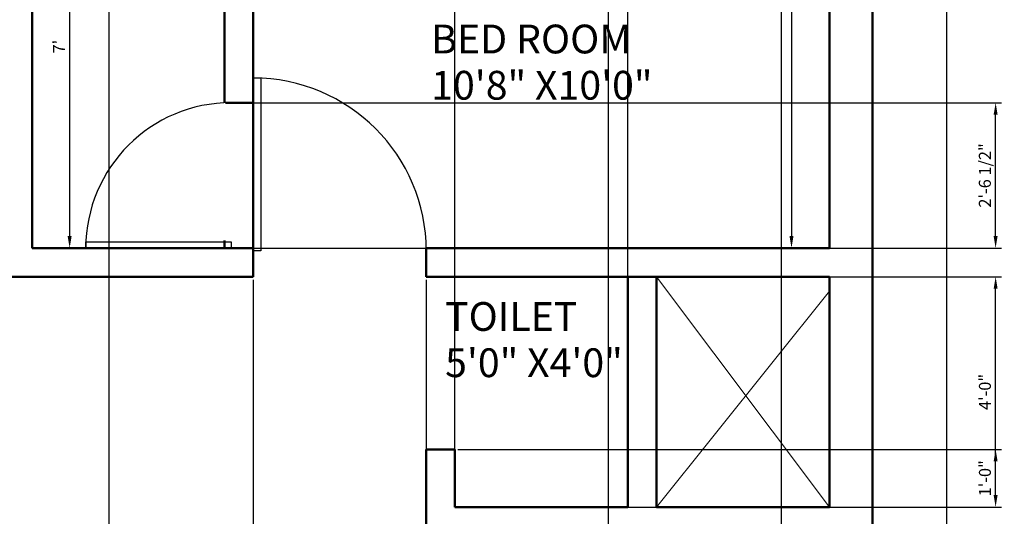
# Model space of a CAD drawing. Units: inches. Extents: x 2385 to 2740, y 1752 to 2305.
# Tile 12 of 15: x 2535 to 2740, y 2091 to 2195. Entities that reach past the tile are written whole.
import ezdxf

# ---------------------------------------------------------------- set-up
doc = ezdxf.new("R2010")
doc.units = ezdxf.units.IN
for name, color, linetype, lineweight in [('A-ANNO-DIMS', 2, 'Continuous', 18), ('A-AREA-IDEN', 7, 'Continuous', 25), ('A-DOOR', 4, 'Continuous', 25), ('A-FLOR-OPEN', 8, 'Continuous', 18), ('A-WALL', 7, 'Continuous', 50)]:
    doc.layers.add(name, color=color, linetype=linetype, lineweight=lineweight)
doc.styles.get("Standard").update_dxf_attribs({"font": 'arial.ttf'})
doc.dimstyles.new('Copy of ISO-25', dxfattribs={"dimtxt": 2.5, "dimasz": 2.5, "dimexe": 1.25, "dimexo": 0.625, "dimtad": 1, "dimdec": 1, "dimlunit": 4, "dimtxsty": 'Standard', "dimcen": 2.5, "dimadec": 0, "dimazin": 0, "dimtfac": 1, "dimtdec": 1, "dimtmove": 0, "dimatfit": 3, "dimfxl": 1, "dimarcsym": 0})

# ---------------------------------------------------------------- blocks, each defined once
blk = doc.blocks.new('*U4')
for p, q in [((0, 0), (0, -6)), ((40, 0), (40, -6))]:
    blk.add_line(p, q)
blk.add_lwpolyline([(0, 0), (0, 40), (1.75, 40), (1.75, 0)], close=True)
blk.add_arc((0, 0), 40, 0, 90)
blk = doc.blocks.new('*U5')
for p, q in [((-40, 0), (-40, 6)), ((0, 0), (0, 6))]:
    blk.add_line(p, q)
blk.add_lwpolyline([(0, 0), (0, -40), (-1.75, -40), (-1.75, 0)], close=True)
blk.add_arc((0, 0), 40, 180, 270)
blk = doc.blocks.new('*D9')
at = {"layer": 'A-ANNO-DIMS', "color": 0, "lineweight": -2, "transparency": 16777216}
for p, q in [((2702.62, 2266.97), (2694.11, 2266.97)), ((2695.36, 2264.47), (2695.36, 2149.47)), ((2702.62, 2146.97), (2694.11, 2146.97))]:
    blk.add_line(p, q, dxfattribs=at)
at = {"layer": 'A-ANNO-DIMS', "color": 0, "transparency": 16777216}
for points in [[(2694.94, 2264.47), (2695.77, 2264.47), (2695.36, 2266.97)], [(2694.94, 2149.47), (2695.77, 2149.47), (2695.36, 2146.97)]]:
    blk.add_solid(points, dxfattribs=at)
at = {"layer": 'Defpoints', "color": 0, "transparency": 16777216}
for p in [(2703.25, 2266.97), (2695.36, 2146.97), (2703.25, 2146.97)]:
    blk.add_point(p, dxfattribs=at)
at = {"layer": 'A-ANNO-DIMS', "color": 0, "transparency": 16777216, "insert": (2693.45, 2206.97), "char_height": 2.5, "attachment_point": 5, "rotation": 90}
blk.add_mtext("10'", dxfattribs=at)
blk = doc.blocks.new('*D11')
at = {"layer": 'A-ANNO-DIMS', "color": 0, "lineweight": -2, "transparency": 16777216}
for p, q in [((2537.87, 2230.97), (2546.28, 2230.97)), ((2545.03, 2228.47), (2545.03, 2149.47)), ((2537.87, 2146.97), (2546.28, 2146.97))]:
    blk.add_line(p, q, dxfattribs=at)
at = {"layer": 'A-ANNO-DIMS', "color": 0, "transparency": 16777216}
for points in [[(2544.61, 2228.47), (2545.44, 2228.47), (2545.03, 2230.97)], [(2544.61, 2149.47), (2545.44, 2149.47), (2545.03, 2146.97)]]:
    blk.add_solid(points, dxfattribs=at)
at = {"layer": 'Defpoints', "color": 0, "transparency": 16777216}
for p in [(2537.25, 2230.97), (2537.25, 2146.97), (2545.03, 2146.97)]:
    blk.add_point(p, dxfattribs=at)
at = {"layer": 'A-ANNO-DIMS', "color": 0, "transparency": 16777216, "insert": (2543.15, 2188.97), "char_height": 2.5, "attachment_point": 5, "rotation": 90}
blk.add_mtext("7'", dxfattribs=at)
blk = doc.blocks.new('*D25')
at = {"layer": 'A-ANNO-DIMS', "color": 0, "lineweight": -2, "transparency": 16777216}
for p, q in [((2712.87, 2275.97), (2728.93, 2275.97)), ((2727.68, 1781.47), (2727.68, 2273.47)), ((2712.87, 1778.97), (2728.93, 1778.97))]:
    blk.add_line(p, q, dxfattribs=at)
at = {"layer": 'A-ANNO-DIMS', "color": 0, "transparency": 16777216}
for points in [[(2727.26, 2273.47), (2728.09, 2273.47), (2727.68, 2275.97)], [(2727.26, 1781.47), (2728.09, 1781.47), (2727.68, 1778.97)]]:
    blk.add_solid(points, dxfattribs=at)
at = {"layer": 'Defpoints', "color": 0, "transparency": 16777216}
for p in [(2712.25, 2275.97), (2727.68, 2275.97), (2712.25, 1778.97)]:
    blk.add_point(p, dxfattribs=at)
at = {"layer": 'A-ANNO-DIMS', "color": 0, "transparency": 16777216, "insert": (2725.77, 2027.47), "char_height": 2.5, "attachment_point": 5, "rotation": 90}
blk.add_mtext('41\'-5"', dxfattribs=at)
blk = doc.blocks.new('*D32')
at = {"layer": 'A-ANNO-DIMS', "color": 0, "lineweight": -2, "transparency": 16777216}
for p, q in [((2625.25, 2093.59), (2625.25, 2302.84)), ((2661.25, 2093.59), (2661.25, 2302.84)), ((2627.75, 2301.59), (2658.75, 2301.59))]:
    blk.add_line(p, q, dxfattribs=at)
at = {"layer": 'A-ANNO-DIMS', "color": 0, "transparency": 16777216}
for points in [[(2627.75, 2302), (2627.75, 2301.17), (2625.25, 2301.59)], [(2658.75, 2302), (2658.75, 2301.17), (2661.25, 2301.59)]]:
    blk.add_solid(points, dxfattribs=at)
at = {"layer": 'Defpoints', "color": 0, "transparency": 16777216}
for p in [(2661.25, 2301.59), (2625.25, 2092.97), (2661.25, 2092.97)]:
    blk.add_point(p, dxfattribs=at)
at = {"layer": 'A-ANNO-DIMS', "color": 0, "transparency": 16777216, "insert": (2643.25, 2303.49), "char_height": 2.5, "attachment_point": 5}
blk.add_mtext('3\'-0"', dxfattribs=at)
blk = doc.blocks.new('*D33')
at = {"layer": 'A-ANNO-DIMS', "color": 0, "lineweight": -2, "transparency": 16777216}
for p, q in [((2661.87, 2140.97), (2739.12, 2140.97)), ((2737.87, 2095.47), (2737.87, 2138.47)), ((2661.87, 2092.97), (2739.12, 2092.97))]:
    blk.add_line(p, q, dxfattribs=at)
at = {"layer": 'A-ANNO-DIMS', "color": 0, "transparency": 16777216}
for points in [[(2737.45, 2138.47), (2738.28, 2138.47), (2737.87, 2140.97)], [(2737.45, 2095.47), (2738.28, 2095.47), (2737.87, 2092.97)]]:
    blk.add_solid(points, dxfattribs=at)
at = {"layer": 'Defpoints', "color": 0, "transparency": 16777216}
for p in [(2661.25, 2140.97), (2737.87, 2140.97), (2661.25, 2092.97)]:
    blk.add_point(p, dxfattribs=at)
at = {"layer": 'A-ANNO-DIMS', "color": 0, "transparency": 16777216, "insert": (2735.96, 2116.97), "char_height": 2.5, "attachment_point": 5, "rotation": 90}
blk.add_mtext('4\'-0"', dxfattribs=at)
blk = doc.blocks.new('*D38')
at = {"layer": 'A-ANNO-DIMS', "color": 0, "lineweight": -2, "transparency": 16777216}
for p, q in [((2577.87, 2177.26), (2739.12, 2177.26)), ((2737.87, 2149.47), (2737.87, 2174.76)), ((2577.87, 2146.97), (2739.12, 2146.97))]:
    blk.add_line(p, q, dxfattribs=at)
at = {"layer": 'A-ANNO-DIMS', "color": 0, "transparency": 16777216}
for points in [[(2737.45, 2174.76), (2738.28, 2174.76), (2737.87, 2177.26)], [(2737.45, 2149.47), (2738.28, 2149.47), (2737.87, 2146.97)]]:
    blk.add_solid(points, dxfattribs=at)
at = {"layer": 'Defpoints', "color": 0, "transparency": 16777216}
for p in [(2577.25, 2177.26), (2737.87, 2177.26), (2577.25, 2146.97)]:
    blk.add_point(p, dxfattribs=at)
at = {"layer": 'A-ANNO-DIMS', "color": 0, "transparency": 16777216, "insert": (2735.95, 2162.11), "char_height": 2.5, "attachment_point": 5, "rotation": 90}
blk.add_mtext('2\'-6 1/2"', dxfattribs=at)
blk = doc.blocks.new('*D43')
at = {"layer": 'A-ANNO-DIMS', "color": 0, "lineweight": -2, "transparency": 16777216}
for p, q in [((2657.25, 1863.59), (2657.25, 2302.84)), ((2693.25, 1863.59), (2693.25, 2302.84)), ((2659.75, 2301.59), (2690.75, 2301.59))]:
    blk.add_line(p, q, dxfattribs=at)
at = {"layer": 'A-ANNO-DIMS', "color": 0, "transparency": 16777216}
for points in [[(2659.75, 2302), (2659.75, 2301.17), (2657.25, 2301.59)], [(2690.75, 2302), (2690.75, 2301.17), (2693.25, 2301.59)]]:
    blk.add_solid(points, dxfattribs=at)
at = {"layer": 'Defpoints', "color": 0, "transparency": 16777216}
for p in [(2693.25, 2301.59), (2657.25, 1862.97), (2693.25, 1862.97)]:
    blk.add_point(p, dxfattribs=at)
at = {"layer": 'A-ANNO-DIMS', "color": 0, "transparency": 16777216, "insert": (2675.25, 2303.49), "char_height": 2.5, "attachment_point": 5}
blk.add_mtext('3\'-0"', dxfattribs=at)
blk = doc.blocks.new('*D44')
at = {"layer": 'A-ANNO-DIMS', "color": 0, "lineweight": -2, "transparency": 16777216}
for p, q in [((2583.25, 2140.34), (2583.25, 1752.1)), ((2619.25, 2140.34), (2619.25, 1752.1)), ((2585.75, 1753.35), (2616.75, 1753.35))]:
    blk.add_line(p, q, dxfattribs=at)
at = {"layer": 'A-ANNO-DIMS', "color": 0, "transparency": 16777216}
for points in [[(2585.75, 1753.77), (2585.75, 1752.94), (2583.25, 1753.35)], [(2616.75, 1753.77), (2616.75, 1752.94), (2619.25, 1753.35)]]:
    blk.add_solid(points, dxfattribs=at)
at = {"layer": 'Defpoints', "color": 0, "transparency": 16777216}
for p in [(2583.25, 2140.97), (2619.25, 2140.97), (2619.25, 1753.35)]:
    blk.add_point(p, dxfattribs=at)
at = {"layer": 'A-ANNO-DIMS', "color": 0, "transparency": 16777216, "insert": (2601.25, 1755.25), "char_height": 2.5, "attachment_point": 5}
blk.add_mtext('3\'-0"', dxfattribs=at)
blk = doc.blocks.new('*D45')
at = {"layer": 'A-ANNO-DIMS', "color": 0, "lineweight": -2, "transparency": 16777216}
for p, q in [((2625.87, 2104.97), (2739.12, 2104.97)), ((2737.87, 2095.47), (2737.87, 2102.47)), ((2625.87, 2092.97), (2739.12, 2092.97))]:
    blk.add_line(p, q, dxfattribs=at)
at = {"layer": 'A-ANNO-DIMS', "color": 0, "transparency": 16777216}
for points in [[(2737.45, 2102.47), (2738.28, 2102.47), (2737.87, 2104.97)], [(2737.45, 2095.47), (2738.28, 2095.47), (2737.87, 2092.97)]]:
    blk.add_solid(points, dxfattribs=at)
at = {"layer": 'Defpoints', "color": 0, "transparency": 16777216}
for p in [(2625.25, 2104.97), (2737.87, 2104.97), (2625.25, 2092.97)]:
    blk.add_point(p, dxfattribs=at)
at = {"layer": 'A-ANNO-DIMS', "color": 0, "transparency": 16777216, "insert": (2735.96, 2098.97), "char_height": 2.5, "attachment_point": 5, "rotation": 90}
blk.add_mtext('1\'-0"', dxfattribs=at)
blk = doc.blocks.new('*D48')
at = {"layer": 'A-ANNO-DIMS', "color": 0, "lineweight": -2, "transparency": 16777216}
for p, q in [((2517.25, 1916.59), (2517.25, 2302.84)), ((2553.25, 1916.59), (2553.25, 2302.84)), ((2519.75, 2301.59), (2550.75, 2301.59))]:
    blk.add_line(p, q, dxfattribs=at)
at = {"layer": 'A-ANNO-DIMS', "color": 0, "transparency": 16777216}
for points in [[(2519.75, 2302), (2519.75, 2301.17), (2517.25, 2301.59)], [(2550.75, 2302), (2550.75, 2301.17), (2553.25, 2301.59)]]:
    blk.add_solid(points, dxfattribs=at)
at = {"layer": 'Defpoints', "color": 0, "transparency": 16777216}
for p in [(2553.25, 2301.59), (2517.25, 1915.97), (2553.25, 1915.97)]:
    blk.add_point(p, dxfattribs=at)
at = {"layer": 'A-ANNO-DIMS', "color": 0, "transparency": 16777216, "insert": (2535.25, 2303.49), "char_height": 2.5, "attachment_point": 5}
blk.add_mtext('3\'-0"', dxfattribs=at)

msp = doc.modelspace()

# ---------------------------------------------------------------- linework, layer by layer
at = {"layer": 'A-FLOR-OPEN'}
for p, q in [((2667.25, 2140.97), (2703.25, 2092.97)), ((2667.25, 2092.97), (2703.25, 2137.97))]:
    msp.add_line(p, q, dxfattribs=at)
at = {"layer": 'A-WALL'}
for p, q in [((2712.25, 2275.97), (2712.25, 2134.97)), ((2712.25, 2275.97), (2712.25, 1778.97)), ((2537.25, 2266.97), (2537.25, 2146.97)), ((2577.25, 2266.97), (2577.25, 2182.97)), ((2583.25, 2182.97), (2583.25, 2266.97)), ((2703.25, 2266.97), (2703.25, 2146.97)), ((2537.25, 2146.97), (2537.25, 2230.97)), ((2577.25, 2182.64), (2577.25, 2182.97)), ((2577.25, 2182.64), (2577.25, 2177.26)), ((2583.25, 2182.97), (2583.25, 2182.65)), ((2583.25, 2182.65), (2583.25, 2146.97)), ((2577.48, 2177.26), (2583.25, 2177.26)), ((2577.25, 2146.97), (2537.25, 2146.97)), ((2577.25, 2146.97), (2577.25, 2148.53)), ((2583.25, 2146.97), (2577.25, 2146.97)), ((2583.25, 2146.97), (2577.25, 2146.97)), ((2583.25, 2146.97), (2583.25, 2140.97)), ((2703.25, 2146.97), (2619.25, 2146.97)), ((2619.25, 2140.97), (2619.25, 2146.97)), ((2583.25, 2140.97), (2531.25, 2140.97)), ((2643.25, 2140.97), (2619.25, 2140.97)), ((2625.25, 2140.97), (2661.25, 2140.97)), ((2643.25, 2140.97), (2652.25, 2140.97)), ((2703.25, 2140.97), (2652.25, 2140.97)), ((2661.25, 2140.97), (2661.25, 2092.97)), ((2667.25, 2092.97), (2667.25, 2140.97)), ((2703.25, 2134.97), (2703.25, 2140.97)), ((2703.25, 2134.97), (2703.25, 2092.97)), ((2712.25, 2134.97), (2712.25, 2086.97)), ((2619.25, 2104.97), (2619.25, 2092.97)), ((2625.25, 2104.97), (2619.25, 2104.97)), ((2625.25, 2092.97), (2625.25, 2104.97)), ((2619.25, 2092.97), (2619.25, 2086.97)), ((2625.25, 2092.97), (2643.25, 2092.97)), ((2643.25, 2092.97), (2652.25, 2092.97)), ((2652.25, 2092.97), (2661.25, 2092.97)), ((2667.25, 2092.97), (2703.25, 2092.97))]:
    msp.add_line(p, q, dxfattribs=at)

# ---------------------------------------------------------------- block references
at = {"layer": 'A-DOOR', "xscale": 0.901135414682081, "yscale": 0.901135414682081, "zscale": 0.901135414682081}
msp.add_blockref('*U4', (2583.25, 2146.38), dxfattribs=at)
at = {"layer": 'A-DOOR', "xscale": 0.7578052513797602, "yscale": 0.7578052513797602, "zscale": 0.7578052513797602, "rotation": 270}
msp.add_blockref('*U5', (2578.7, 2146.97), dxfattribs=at)

# ---------------------------------------------------------------- texts
at = {"layer": 'A-AREA-IDEN'}
for s, p in [('BED ROOM', (2620.32, 2187.55)), ('10\'8" X10\'0"', (2620.32, 2177.91)), ('TOILET', (2623.22, 2129.7)), ('5\'0" X4\'0"', (2623.22, 2120.06))]:
    msp.add_text(s, height=6, dxfattribs=at).set_placement(p)

# ---------------------------------------------------------------- dimensions: what is measured, and where the dimension line sits
at = {"layer": 'A-ANNO-DIMS'}
for base, p1, p2, picture, middle in [((2553.25, 2301.59), (2517.25, 1915.97), (2553.25, 1915.97), '*D48', (2535.25, 2303.49)), ((2661.25, 2301.59), (2625.25, 2092.97), (2661.25, 2092.97), '*D32', (2643.25, 2303.49)), ((2693.25, 2301.59), (2657.25, 1862.97), (2693.25, 1862.97), '*D43', (2675.25, 2303.49)), ((2619.25, 1753.35), (2583.25, 2140.97), (2619.25, 2140.97), '*D44', (2601.25, 1755.25))]:
    dim = msp.add_linear_dim(base=base, p1=p1, p2=p2, dimstyle='Copy of ISO-25', override={"dimdec": 1, "dimlfac": 1, "dimrnd": 0, "dimzin": 1, "dimdsep": 46, "dimlunit": 4, "dimfrac": 2}, dxfattribs=at)
    dim.commit()
    dim.dimension.update_dxf_attribs({"geometry": picture, "text_midpoint": middle})
for base, p1, p2, override, picture, middle in [((2727.68, 2275.97), (2712.25, 1778.97), (2712.25, 2275.97), {"dimclrd": 0, "dimclre": 0, "dimclrt": 0}, '*D25', (2725.77, 2027.47)), ((2695.36, 2146.97), (2703.25, 2266.97), (2703.25, 2146.97), {"dimclrd": 0, "dimclre": 0, "dimclrt": 0}, '*D9', (2693.45, 2206.97)), ((2545.03, 2146.97), (2537.25, 2230.97), (2537.25, 2146.97), {"dimclrd": 0, "dimclre": 0, "dimclrt": 0}, '*D11', (2543.15, 2188.97)), ((2737.87, 2177.26), (2577.25, 2146.97), (2577.25, 2177.26), {"dimdec": 1, "dimlfac": 1, "dimrnd": 0, "dimzin": 1, "dimdsep": 46, "dimlunit": 4, "dimfrac": 2}, '*D38', (2735.95, 2162.11)), ((2737.87, 2140.97), (2661.25, 2092.97), (2661.25, 2140.97), {"dimdec": 1, "dimlfac": 1, "dimrnd": 0, "dimzin": 1, "dimdsep": 46, "dimlunit": 4, "dimfrac": 2}, '*D33', (2735.96, 2116.97)), ((2737.87, 2104.97), (2625.25, 2092.97), (2625.25, 2104.97), {"dimdec": 1, "dimlfac": 1, "dimrnd": 0, "dimzin": 1, "dimdsep": 46, "dimlunit": 4, "dimfrac": 2}, '*D45', (2735.96, 2098.97))]:
    dim = msp.add_linear_dim(base=base, p1=p1, p2=p2, angle=90, dimstyle='Copy of ISO-25', override=override, dxfattribs=at)
    dim.commit()
    dim.dimension.update_dxf_attribs({"geometry": picture, "text_midpoint": middle})

doc.saveas('drawing.dxf')
